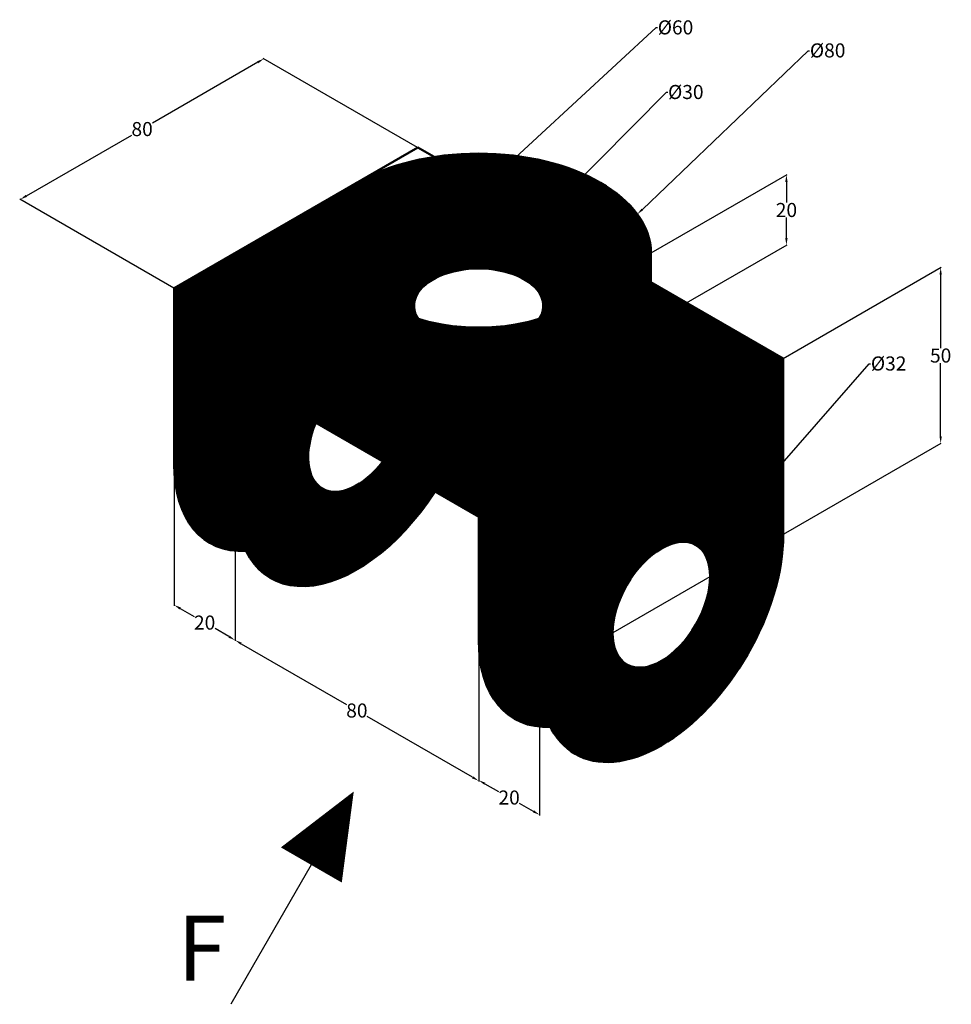
# Model space of a CAD drawing. Units: millimetres. Extents: x -475 to 40, y -900 to -205.
# Tile 1 of 1: x -318.9 to -53.9, y -485 to -205. Entities that reach past the tile are written whole.
import ezdxf
from ezdxf import colors
from ezdxf.entities.mleader import LeaderData, LeaderLine
from ezdxf.math import Vec2, Vec3

# ---------------------------------------------------------------- set-up
doc = ezdxf.new("R2010")
doc.units = ezdxf.units.MM
doc.header["$MEASUREMENT"] = 0
for name, color, linetype, lineweight in [('M-ANNO-SYMB', 2, 'Continuous', 25), ('M-DIMS', 2, 'Continuous', 25), ('M-HATC', 8, 'Continuous', 18), ('M-OUTL', 7, 'Continuous', 50), ('M-TEXT', 7, 'Continuous', 25)]:
    doc.layers.add(name, color=color, linetype=linetype, lineweight=lineweight)
doc.styles.get("Standard").update_dxf_attribs({"font": 'arial.ttf'})
doc.dimstyles.get("Standard").update_dxf_attribs({"dimtxt": 4, "dimasz": 2, "dimexe": 0.18, "dimexo": 0.0625, "dimgap": 0.09, "dimtad": 0, "dimtih": 1, "dimtoh": 1, "dimdec": 0, "dimzin": 0, "dimdsep": 46, "dimtxsty": 'Standard', "dimcen": 0.09, "dimadec": 0, "dimazin": 0, "dimtfac": 1, "dimtdec": 0, "dimtofl": 0, "dimtmove": 0, "dimatfit": 3, "dimfxl": 1, "dimtolj": 1, "dimtzin": 0, "dimarcsym": 0})

# ---------------------------------------------------------------- blocks, each defined once
blk = doc.blocks.new('*D1')
at = {"layer": 'Defpoints', "color": 0, "transparency": 16777216}
for p in [(-56.94566817318142, -325.4711766746398), (-171.0183611883869, -341.3310766941546), (-171.0183611883869, -391.3310766941547)]:
    blk.add_point(p, dxfattribs=at)
at = {"layer": 'M-DIMS', "color": 0, "lineweight": -2, "transparency": 16777216}
for p, q in [((-170.9558611883869, -341.2949923023302), (-56.76566817318142, -275.3672536261856)), ((-56.94566817318142, -277.4711766746397), (-56.94566817318142, -298.3388847237529)), ((-56.94566817318142, -323.4711766746398), (-56.94566817318142, -302.6034686255265)), ((-170.9558611883869, -391.2949923023303), (-56.76566817318141, -325.3672536261856))]:
    blk.add_line(p, q, dxfattribs=at)
at = {"layer": 'M-DIMS', "color": 0, "transparency": 16777216}
for points in [[(-57.27900150651476, -277.4711766746397), (-56.61233483984808, -277.4711766746397), (-56.94566817318142, -275.4711766746397)], [(-57.27900150651475, -323.4711766746398), (-56.61233483984808, -323.4711766746398), (-56.94566817318142, -325.4711766746398)]]:
    blk.add_solid(points, dxfattribs=at)
at = {"layer": 'M-DIMS', "color": 0, "transparency": 16777216, "insert": (-56.9456681731815, -300.4711766746396), "char_height": 4, "attachment_point": 5}
blk.add_mtext('\\A1;50', dxfattribs=at)
blk = doc.blocks.new('*D2')
at = {"layer": 'Defpoints', "color": 0, "transparency": 16777216}
for p in [(-188.3388692640756, -346.3310766941546), (-171.0183611883868, -356.164245815369), (-171.0183611883869, -431.07672200079)]:
    blk.add_point(p, dxfattribs=at)
at = {"layer": 'M-DIMS', "color": 0, "lineweight": -2, "transparency": 16777216}
for p, q in [((-188.3388692640756, -346.402946369226), (-188.3388692640757, -421.4505375437814)), ((-171.0183611883868, -356.2361154904404), (-171.0183611883869, -431.2837066649958)), ((-186.5996099745945, -422.2309621786778), (-182.6608389642941, -424.4670744973681)), ((-172.757620477868, -430.0893127016877), (-176.6963914881685, -427.8532003829974))]:
    blk.add_line(p, q, dxfattribs=at)
at = {"layer": 'M-DIMS', "color": 0, "transparency": 16777216}
for points in [[(-186.4350417580775, -421.941085630431), (-186.7641781911116, -422.5208387269247), (-188.3388692640757, -421.2435528795755)], [(-172.5930522613509, -429.7994361534409), (-172.922188694385, -430.3791892499345), (-171.0183611883869, -431.07672200079)]]:
    blk.add_solid(points, dxfattribs=at)
at = {"layer": 'M-DIMS', "color": 0, "transparency": 16777216, "insert": (-179.6786152262312, -426.1601374401827), "char_height": 4, "attachment_point": 5}
blk.add_mtext('\\A1;20', dxfattribs=at)
blk = doc.blocks.new('*D3')
at = {"layer": 'Defpoints', "color": 0, "transparency": 16777216}
for p in [(-257.6209015668307, -341.3310766941545), (-257.6209015668307, -381.4107159153928), (-188.3388692640756, -381.3310766941545)]:
    blk.add_point(p, dxfattribs=at)
at = {"layer": 'M-DIMS', "color": 0, "lineweight": -2, "transparency": 16777216}
for p, q in [((-257.6209015668307, -341.4032454778032), (-257.6209015668307, -381.618562012301)), ((-255.8888507592618, -382.4107159153927), (-225.9307312544708, -399.7070442758987)), ((-188.3388692640756, -381.4032454778032), (-188.3388692640756, -421.618562012301)), ((-190.0709200716445, -420.4107159153927), (-220.0290395764354, -403.1143875548867))]:
    blk.add_line(p, q, dxfattribs=at)
at = {"layer": 'M-DIMS', "color": 0, "transparency": 16777216}
for points in [[(-255.7221840925951, -382.1220407807979), (-256.0555174259284, -382.6993910499875), (-257.6209015668307, -381.4107159153928)], [(-189.9042534049778, -420.1220407807979), (-190.2375867383111, -420.6993910499875), (-188.3388692640756, -421.4107159153927)]]:
    blk.add_solid(points, dxfattribs=at)
at = {"layer": 'M-DIMS', "color": 0, "transparency": 16777216, "insert": (-222.9798854154531, -401.4107159153927), "char_height": 4, "attachment_point": 5}
blk.add_mtext('\\A1;80', dxfattribs=at)
blk = doc.blocks.new('*D4')
at = {"layer": 'Defpoints', "color": 0, "transparency": 16777216}
for p in [(-274.9414096425195, -331.3310766941545), (-257.6209015668307, -341.3310766941545), (-274.9414096425194, -371.4107159153929)]:
    blk.add_point(p, dxfattribs=at)
at = {"layer": 'M-DIMS', "color": 0, "lineweight": -2, "transparency": 16777216}
for p, q in [((-274.9414096425195, -331.4032454778032), (-274.9414096425194, -371.6185620123011)), ((-257.6209015668307, -341.4032454778032), (-257.6209015668307, -381.6185620123011)), ((-273.2093588349505, -372.4107159153929), (-269.2633793427378, -374.6889282374386)), ((-259.3529523743995, -380.4107159153929), (-263.2989318666123, -378.1325035933471))]:
    blk.add_line(p, q, dxfattribs=at)
at = {"layer": 'M-DIMS', "color": 0, "transparency": 16777216}
for points in [[(-273.0426921682839, -372.122040780798), (-273.3760255016172, -372.6993910499877), (-274.9414096425194, -371.4107159153929)], [(-259.1862857077329, -380.122040780798), (-259.5196190410662, -380.6993910499877), (-257.6209015668307, -381.4107159153929)]]:
    blk.add_solid(points, dxfattribs=at)
at = {"layer": 'M-DIMS', "color": 0, "transparency": 16777216, "insert": (-266.2811556046751, -376.4107159153929), "char_height": 4, "attachment_point": 5}
blk.add_mtext('\\A1;20', dxfattribs=at)
blk = doc.blocks.new('*D5')
at = {"layer": 'Defpoints', "color": 0, "transparency": 16777216}
for p in [(-249.4178865535401, -216.0670896202445), (-205.6593773397644, -241.3310766941545), (-274.9414096425195, -281.3310766941545)]:
    blk.add_point(p, dxfattribs=at)
at = {"layer": 'M-DIMS', "color": 0, "lineweight": -2, "transparency": 16777216}
for p, q in [((-251.149937361109, -217.0670896202445), (-281.1080568658999, -234.3634179807505)), ((-205.7218773397644, -241.2949923023302), (-249.5978865535401, -215.9631665717903)), ((-316.9678680487263, -255.0670896202445), (-287.0097485439354, -237.7707612597385)), ((-275.0039096425195, -281.2949923023302), (-318.8799188562951, -255.9631665717903))]:
    blk.add_line(p, q, dxfattribs=at)
at = {"layer": 'M-DIMS', "color": 0, "transparency": 16777216}
for points in [[(-251.3166040277756, -216.7784144856497), (-250.9832706944423, -217.3557647548393), (-249.4178865535401, -216.0670896202445)], [(-317.134534715393, -254.7784144856497), (-316.8012013820596, -255.3557647548393), (-318.6999188562952, -256.0670896202445)]]:
    blk.add_solid(points, dxfattribs=at)
at = {"layer": 'M-DIMS', "color": 0, "transparency": 16777216, "insert": (-284.0589027049176, -236.0670896202445), "char_height": 4, "attachment_point": 5}
blk.add_mtext('\\A1;80', dxfattribs=at)
blk = doc.blocks.new('*D6')
at = {"layer": 'Defpoints', "color": 0, "transparency": 16777216}
for p in [(-139.3490744084121, -271.3310766941546), (-100.8156650904446, -269.0838024516319), (-139.3490744084121, -291.3310766941546)]:
    blk.add_point(p, dxfattribs=at)
at = {"layer": 'M-DIMS', "color": 0, "lineweight": -2, "transparency": 16777216}
for p, q in [((-139.2865744084121, -271.2949923023302), (-100.6356650904446, -248.9798794031778)), ((-100.8156650904446, -251.0838024516319), (-100.8156650904446, -256.9515105007451)), ((-100.8156650904446, -267.0838024516319), (-100.8156650904446, -261.2160944025187)), ((-139.2865744084121, -291.2949923023303), (-100.6356650904446, -268.9798794031777))]:
    blk.add_line(p, q, dxfattribs=at)
at = {"layer": 'M-DIMS', "color": 0, "transparency": 16777216}
for points in [[(-101.148998423778, -251.0838024516319), (-100.4823317571113, -251.0838024516319), (-100.8156650904446, -249.0838024516319)], [(-101.148998423778, -267.0838024516319), (-100.4823317571113, -267.0838024516319), (-100.8156650904446, -269.0838024516319)]]:
    blk.add_solid(points, dxfattribs=at)
at = {"layer": 'M-DIMS', "color": 0, "transparency": 16777216, "insert": (-100.8156650904447, -259.0838024516318), "char_height": 4, "attachment_point": 5}
blk.add_mtext('\\A1;20', dxfattribs=at)

msp = doc.modelspace()

# ---------------------------------------------------------------- hatches: boundary and pattern name
at = {"layer": 'M-HATC'}
h = msp.add_hatch(dxfattribs=at)
h.set_pattern_fill('ANSI31', color=256)
h.set_pattern_definition([(45, (-328.3383552602089, -427.0710071446905), (-0.0883883476483185, 0.0883883476483185), [])])
edge = h.paths.add_edge_path()
edge.add_ellipse((-188.3388692640756, -271.3310766941545), major_axis=(-48.98979485566356, 3.1e-15), ratio=0.577350269189626, start_angle=330, end_angle=360, ccw=False)
edge.add_line((-222.9798854154533, -251.3310766941545), (-274.9414096425195, -281.3310766941545))
edge.add_line((-274.9414096425195, -281.3310766941545), (-222.979885415453, -311.3310766941546))
edge.add_ellipse((-188.3388692640756, -291.3310766941545), major_axis=(-48.98979485566356, 3.1e-15), ratio=0.577350269189626, start_angle=0, end_angle=30, ccw=False)
edge.add_line((-237.3286641197392, -291.3310766941545), (-237.3286641197392, -271.3310766941545))
edge = h.paths.add_edge_path()
edge.add_line((-101.7363288856317, -301.3310766941545), (-139.349074408412, -279.6153479416164))
edge.add_line((-139.349074408412, -279.6153479416164), (-139.349074408412, -291.3310766941543))
edge.add_ellipse((-188.3388692640756, -291.3310766941545), major_axis=(-48.98979485566356, 3.1e-15), ratio=0.577350269189626, start_angle=30, end_angle=180, ccw=False)
edge.add_line((-222.9798854154533, -311.3310766941544), (-171.0183611883868, -341.3310766941545))
edge.add_line((-171.0183611883868, -341.3310766941545), (-101.7363288856317, -301.3310766941545))
edge = h.paths.add_edge_path()
edge.add_ellipse((-188.3388692640756, -291.3310766941545), major_axis=(-48.98979485566356, 3.1e-15), ratio=0.577350269189626, start_angle=30.00000000000002, end_angle=180)
edge.add_line((-139.349074408412, -291.3310766941543), (-139.349074408412, -279.6153479416164))
edge.add_line((-139.349074408412, -279.6153479416164), (-139.349074408412, -271.3310766941544))
edge.add_ellipse((-188.3388692640756, -271.3310766941545), major_axis=(-48.98979485566356, 3.1e-15), ratio=0.577350269189626, start_angle=0, end_angle=180, ccw=False)
edge.add_line((-237.3286641197392, -271.3310766941545), (-237.3286641197392, -291.3310766941545))
edge.add_ellipse((-188.3388692640756, -291.3310766941545), major_axis=(-48.98979485566356, 3.1e-15), ratio=0.577350269189626, start_angle=0, end_angle=30.00000000000002)
edge = h.paths.add_edge_path()
edge.add_ellipse((-188.3388692640756, -271.3310766941545), major_axis=(-48.98979485566356, 3.1e-15), ratio=0.577350269189626, start_angle=3.6e-15, end_angle=180)
edge.add_ellipse((-188.3388692640756, -271.3310766941545), major_axis=(-48.98979485566356, 3.1e-15), ratio=0.577350269189626, start_angle=180, end_angle=216.4273398800309)
edge.add_line((-158.1530337662851, -249.0539184724817), (-164.3185950845215, -255.2788034559799))
edge.add_ellipse((-188.3388692640756, -271.3310766941545), major_axis=(-36.74234614174767, 1.5e-15), ratio=0.577350269189626, start_angle=167.6900113356715, end_angle=213.7540221323888, ccw=False)
edge.add_ellipse((-188.3388692640756, -271.3310766941545), major_axis=(-36.74234614174767, 1.5e-15), ratio=0.577350269189626, start_angle=132.5057290121876, end_angle=167.6900113356715, ccw=False)
edge.add_ellipse((-188.3388692640756, -271.3310766941545), major_axis=(-36.74234614174767, 1.5e-15), ratio=0.577350269189626, start_angle=47.4942709878124, end_angle=132.5057290121876, ccw=False)
edge.add_ellipse((-188.3388692640756, -271.3310766941545), major_axis=(-36.74234614174767, 1.5e-15), ratio=0.577350269189626, start_angle=12.309988664328614, end_angle=47.4942709878124, ccw=False)
edge.add_ellipse((-188.3388692640756, -271.3310766941545), major_axis=(-36.74234614174767, 1.5e-15), ratio=0.577350269189626, start_angle=213.7540221323888, end_angle=372.30998866432856, ccw=False)
edge.add_line((-164.3185950845215, -255.2788034559799), (-158.1530337662851, -249.0539184724817))
edge.add_ellipse((-188.3388692640756, -271.3310766941545), major_axis=(-48.98979485566356, 3.1e-15), ratio=0.577350269189626, start_angle=216.4273398800309, end_angle=248.418359243648)
edge.add_ellipse((-188.3388692640756, -271.3310766941545), major_axis=(-48.98979485566356, 3.1e-15), ratio=0.577350269189626, start_angle=248.418359243648, end_angle=294.8960906389828)
edge.add_ellipse((-188.3388692640756, -271.3310766941545), major_axis=(-48.98979485566356, 3.1e-15), ratio=0.577350269189626, start_angle=294.8960906389828, end_angle=330)
edge.add_ellipse((-188.3388692640756, -271.3310766941545), major_axis=(-48.98979485566356, 3.1e-15), ratio=0.577350269189626, start_angle=330, end_angle=360)
edge = h.paths.add_edge_path(flags=17)
edge.add_ellipse((-188.3388692640756, -271.3310766941545), major_axis=(-36.74234614174767, 1.5e-15), ratio=0.577350269189626, start_angle=213.7540221323888, end_angle=372.3099886643286)
edge.add_ellipse((-188.3388692640756, -286.3310766941545), major_axis=(-36.74234614174767, 1.5e-15), ratio=0.577350269189626, start_angle=236.92679235372322, end_angle=347.69001133567144, ccw=False)
edge.add_line((-175.4080661358342, -266.474974941304), (-164.3185950845215, -255.27880345598))
edge = h.paths.add_edge_path(flags=17)
edge.add_ellipse((-188.3388692640756, -271.3310766941545), major_axis=(-36.74234614174767, 1.5e-15), ratio=0.577350269189626, start_angle=167.6900113356714, end_angle=213.7540221323888)
edge.add_line((-164.3185950845215, -255.2788034559799), (-175.4080661358342, -266.474974941304))
edge.add_ellipse((-188.3388692640756, -286.3310766941545), major_axis=(-36.74234614174767, 1.5e-15), ratio=0.577350269189626, start_angle=192.3099886643282, end_angle=236.9267923537231, ccw=False)
edge = h.paths.add_edge_path(flags=17)
edge.add_ellipse((-188.3388692640756, -286.3310766941545), major_axis=(-36.74234614174767, 1.5e-15), ratio=0.577350269189626, start_angle=192.3099886643282, end_angle=236.9267923537231)
edge.add_ellipse((-188.3388692640756, -286.3310766941545), major_axis=(-36.74234614174767, 1.5e-15), ratio=0.577350269189626, start_angle=236.9267923537231, end_angle=347.6900113356714)
edge.add_ellipse((-188.3388692640756, -271.3310766941545), major_axis=(-36.74234614174767, 1.5e-15), ratio=0.577350269189626, start_angle=12.30998866432856, end_angle=47.49427098781236)
edge.add_ellipse((-188.3388692640756, -286.3310766941545), major_axis=(-18.37117307087383, 1.5e-15), ratio=0.577350269189626, start_angle=167.6900113356715, end_angle=372.30998866432856, ccw=False)
edge.add_ellipse((-188.3388692640756, -271.3310766941545), major_axis=(-36.74234614174767, 1.5e-15), ratio=0.577350269189626, start_angle=132.5057290121876, end_angle=167.6900113356714)
edge = h.paths.add_edge_path()
edge.add_line((-101.7363288856317, -301.3310766941545), (-171.0183611883868, -341.3310766941545))
edge.add_line((-171.0183611883868, -341.3310766941545), (-171.0183611883868, -391.3310766941542))
edge.add_ellipse((-136.3773450370093, -371.3310766941545), major_axis=(-24.49489742783177, -42.42640687119285), ratio=0.577350269189626, start_angle=329.9999999999999, end_angle=347.6900113356714)
edge.add_ellipse((-136.3773450370093, -371.3310766941545), major_axis=(-24.49489742783177, -42.42640687119285), ratio=0.577350269189626, start_angle=347.6900113356714, end_angle=509.9999999999999)
edge.add_line((-101.7363288856317, -351.3310766941553), (-101.7363288856317, -301.3310766941545))
edge = h.paths.add_edge_path(flags=16)
edge.add_ellipse((-136.3773450370093, -371.3310766941545), major_axis=(-9.797958971132706, -16.97056274847714), ratio=0.577350269189626, start_angle=0, end_angle=360)
edge = h.paths.add_edge_path()
edge.add_line((-222.9798854154533, -311.3310766941544), (-274.9414096425195, -281.3310766941545))
edge.add_line((-274.9414096425195, -281.3310766941545), (-274.9414096425195, -331.3310766941543))
edge.add_ellipse((-240.3003934911419, -311.3310766941545), major_axis=(-24.49489742783177, -42.42640687119285), ratio=0.577350269189626, start_angle=329.9999999999999, end_angle=372.3099886642788)
edge.add_ellipse((-222.9798854154532, -321.3310766941545), major_axis=(-24.49489742783177, -42.42640687119285), ratio=0.577350269189626, start_angle=329.99999999999994, end_angle=347.69001133567144, ccw=False)
edge.add_line((-257.6209015668307, -341.3310766941541), (-257.6209015668307, -306.3310766941545))
edge.add_line((-257.6209015668307, -306.3310766941545), (-188.3388692640756, -346.3310766941545))
edge.add_line((-188.3388692640756, -346.3310766941545), (-188.3388692640756, -381.3310766941543))
edge.add_ellipse((-153.697853112698, -361.3310766941545), major_axis=(-24.49489742783177, -42.42640687119285), ratio=0.577350269189626, start_angle=329.9999999999999, end_angle=372.3099886642788)
edge.add_ellipse((-136.3773450370093, -371.3310766941545), major_axis=(-24.49489742783177, -42.42640687119285), ratio=0.577350269189626, start_angle=329.99999999999994, end_angle=347.69001133567144, ccw=False)
edge.add_line((-171.0183611883868, -391.331076694154), (-171.0183611883868, -341.3310766941545))
edge.add_line((-171.0183611883868, -341.3310766941545), (-222.9798854154533, -311.3310766941544))
edge = h.paths.add_edge_path(flags=17)
edge.add_ellipse((-222.9798854154532, -321.3310766941545), major_axis=(-24.49489742783177, -42.42640687119285), ratio=0.577350269189626, start_angle=347.6900113356714, end_angle=441.2623174267488)
edge.add_line((-200.7459223049853, -339.1678612811353), (-215.5891914981061, -330.5980958168329))
edge.add_ellipse((-222.9798854154532, -321.3310766941545), major_axis=(-9.797958971132706, -16.97056274847714), ratio=0.577350269189626, start_angle=291.4267091514603, end_angle=428.5732908485397, ccw=False)
edge.add_line((-234.7007063517224, -319.564057571476), (-257.6209015668307, -306.3310766941545))
edge.add_line((-257.6209015668307, -306.3310766941545), (-257.6209015668307, -341.3310766941541))
edge.add_ellipse((-222.9798854154532, -321.3310766941545), major_axis=(-24.49489742783177, -42.42640687119285), ratio=0.577350269189626, start_angle=329.9999999999999, end_angle=347.6900113356714)

# ---------------------------------------------------------------- linework, layer by layer
at = {"layer": 'M-ANNO-SYMB'}
msp.add_line((-235.9352353405691, -445.3403348579658), (-258.8089789745049, -484.9588209912478), dxfattribs=at)
msp.add_lwpolyline([(-235.9352353405691, -445.3403348579658, 20, 0, 0), (-223.8609380176139, -424.4270384289145, 0, 0, 0)], format="xyseb", dxfattribs=at)
at = {"layer": 'M-OUTL'}
for p, q in [((-274.9414096425195, -281.3310766941545), (-205.6593773397644, -241.3310766941545)), ((-205.6593773397644, -241.3310766941545), (-201.0183611883868, -244.0105686184658)), ((-237.3286641197392, -271.3310766941545), (-237.3286641197392, -291.3310766941545)), ((-139.349074408412, -271.3310766941545), (-139.349074408412, -291.3310766941545)), ((-139.349074408412, -279.6153479416164), (-101.7363288856317, -301.3310766941545)), ((-171.0183611883868, -341.3310766941545), (-274.9414096425195, -281.3310766941545)), ((-274.9414096425195, -281.3310766941545), (-274.9414096425195, -331.3310766941545)), ((-171.0183611883868, -341.3310766941545), (-101.7363288856317, -301.3310766941545)), ((-101.7363288856317, -301.3310766941545), (-101.7363288856317, -351.3310766941545)), ((-257.6209015668307, -306.3310766941545), (-257.6209015668307, -341.3310766941545)), ((-188.3388692640756, -346.3310766941545), (-257.6209015668307, -306.3310766941545)), ((-171.0183611883868, -341.3310766941545), (-171.0183611883868, -391.3310766941545)), ((-188.3388692640756, -346.3310766941545), (-188.3388692640756, -381.3310766941545))]:
    msp.add_line(p, q, dxfattribs=at)
for centre, major_axis in [((-188.3388692640756, -271.3310766941545), (-48.98979485566356, 3.1e-15)), ((-188.3388692640756, -271.3310766941545), (-36.74234614174767, 1.5e-15)), ((-136.3773450370093, -371.3310766941545), (-9.797958971132706, -16.97056274847714))]:
    msp.add_ellipse(centre, major_axis=major_axis, ratio=0.577350269189626, dxfattribs=at)
for centre, major_axis, start_param, end_param in [((-188.3388692640756, -286.3310766941545), (-36.74234614174767, 1.5e-15), 3.50295977749649, 5.921818183272877), ((-188.3388692640756, -286.3310766941545), (-18.37117307087383, 1.5e-15), 2.780225529683085, 6.644552431086293), ((-188.3388692640756, -291.3310766941545), (-48.98979485566356, 3.1e-15), 0, 3.141592653589793), ((-222.9798854154532, -321.3310766941545), (-9.797958971132706, -16.97056274847714), 4.935198815711101, 7.631171798648071), ((-240.3003934911419, -311.3310766941545), (-24.49489742783177, -42.42640687119285), 5.497787143782137, 6.644552431084916), ((-222.9798854154532, -321.3310766941545), (-24.49489742783177, -42.42640687119285), 5.497787143782137, 7.765477790830463), ((-136.3773450370093, -371.3310766941545), (-24.49489742783177, -42.42640687119285), 5.497787143782137, 8.63937979737193), ((-153.697853112698, -361.3310766941545), (-24.49489742783177, -42.42640687119285), 5.497787143782137, 6.644552431084916)]:
    msp.add_ellipse(centre, major_axis=major_axis, ratio=0.577350269189626, start_param=start_param, end_param=end_param, dxfattribs=at)

# ---------------------------------------------------------------- texts
at = {"layer": 'M-TEXT'}
msp.add_text('F', height=18.43271151920555, dxfattribs=at).set_placement((-274.0271530944519, -478.2182776550038))

# ---------------------------------------------------------------- dimensions: what is measured, and where the dimension line sits
at = {"layer": 'M-DIMS'}
for p1, p2, distance, picture, middle in [((-274.9414096425195, -281.3310766941545), (-205.6593773397644, -241.3310766941545), 43.75850921377558, '*D5', (-284.0589027049176, -236.0670896202445)), ((-139.349074408412, -271.3310766941545), (-139.349074408412, -291.3310766941545), 38.53340931796741, '*D6', (-100.8156650904447, -259.0838024516318)), ((-171.0183611883868, -341.3310766941545), (-171.0183611883868, -391.3310766941545), 114.07269301520537, '*D1', (-56.9456681731815, -300.4711766746396)), ((-257.6209015668307, -341.3310766941545), (-274.9414096425195, -331.3310766941545), 34.70998574010759, '*D4', (-266.2811556046751, -376.4107159153929)), ((-188.3388692640756, -381.3310766941545), (-257.6209015668307, -341.3310766941545), 34.70998574010754, '*D3', (-222.9798854154531, -401.4107159153927)), ((-188.3388692640756, -346.3310766941545), (-171.0183611883868, -356.1642458153689), -65.14611005176354, '*D2', (-179.6786152262312, -426.1601374401827))]:
    dim = msp.add_aligned_dim(p1=p1, p2=p2, distance=distance, dimstyle='Standard', override={"dimclrd": 0, "dimclre": 0, "dimclrt": 0}, dxfattribs=at)
    dim.commit()
    dim.dimension.update_dxf_attribs({"geometry": picture, "text_midpoint": middle})

# ---------------------------------------------------------------- leaders
ml = msp.add_multileader_mtext('Standard', dxfattribs=at)
ml.set_content('%%C60', color=256)
ml.set_leader_properties()
ml.build(insert=Vec2(0, 0))
ml.multileader.update_dxf_attribs({"dogleg_length": 0.36, "arrow_head_size": 2})
ctx = ml.context
ctx.base_point, ctx.arrow_head_size, ctx.landing_gap_size, ctx.plane_origin = Vec3(-137.498386941451, -207.2357888024651), 2, 0.09, Vec3(-184.4533055337964, -250.2368247559452)
notes = []
notes.append((ctx, [(0, (1, 1, 0), (-137.858386941451, -207.2357888024651), (1, 0), 0.36, [(0, [(-184.4533055337964, -250.2368247559452)], 0, [])])]))
ctx.mtext.insert, ctx.mtext.flow_direction = Vec3(-137.408386941451, -205.1552976701323), 5
ml = msp.add_multileader_mtext('Standard', dxfattribs=at)
ml.set_content('%%C80', color=256)
ml.set_leader_properties()
ml.build(insert=Vec2(0, 0))
ml.multileader.update_dxf_attribs({"dogleg_length": 0.36, "arrow_head_size": 2})
ctx = ml.context
ctx.base_point, ctx.arrow_head_size, ctx.landing_gap_size, ctx.plane_origin = Vec3(-94.2272415017568, -213.7873324322215), 2, 0.09, Vec3(-143.2340961519432, -260.2923653789229)
notes.append((ctx, [(0, (1, 1, 0), (-94.58724150175681, -213.7873324322215), (1, 0), 0.36, [(0, [(-143.2340961519369, -260.2923653789316)], 0, [])])]))
ctx.mtext.insert, ctx.mtext.flow_direction = Vec3(-94.1372415017568, -211.7068412998886), 5
ml = msp.add_multileader_mtext('Standard', dxfattribs=at)
ml.set_content('%%C30', color=256)
ml.set_leader_properties()
ml.build(insert=Vec2(0, 0))
ml.multileader.update_dxf_attribs({"dogleg_length": 0.36, "arrow_head_size": 2})
ctx = ml.context
ctx.base_point, ctx.arrow_head_size, ctx.landing_gap_size, ctx.plane_origin = Vec3(-134.5767980746226, -225.6143013036554), 2, 0.09, Vec3(-184.769601774938, -275.9265852026401)
notes.append((ctx, [(0, (1, 1, 0), (-134.9367980746226, -225.6143013036554), (1, 0), 0.36, [(0, [(-184.769601774938, -275.9265852026401)], 0, [])])]))
ctx.mtext.insert, ctx.mtext.flow_direction = Vec3(-134.4867980746226, -223.5338101713225), 5
ml = msp.add_multileader_mtext('Standard', dxfattribs=at)
ml.set_content('%%C32', color=256)
ml.set_leader_properties()
ml.build(insert=Vec2(0, 0))
ml.multileader.update_dxf_attribs({"dogleg_length": 0.36, "arrow_head_size": 2})
ctx = ml.context
ctx.base_point, ctx.arrow_head_size, ctx.landing_gap_size, ctx.plane_origin = Vec3(-76.88150865255433, -302.8146716772694), 2, 0.09, Vec3(-124.2355850813548, -356.6114961047599)
notes.append((ctx, [(0, (1, 1, 0), (-77.24150865255433, -302.8146716772694), (1, 0), 0.36, [(0, [(-124.2355850813548, -356.6114961047599)], 0, [])])]))
ctx.mtext.insert, ctx.mtext.flow_direction = Vec3(-76.79150865255433, -300.7341805449365), 5
for ctx, leaders in notes:
    for number, flags, end, landing, length, lines in leaders:
        leader = LeaderData()
        leader.index, (leader.has_last_leader_line, leader.has_dogleg_vector, leader.attachment_direction) = number, flags
        leader.last_leader_point, leader.dogleg_vector, leader.dogleg_length = Vec3(end), Vec3(landing), length
        for number, points, colour, breaks in lines:
            line = LeaderLine()
            line.index, line.vertices, line.color, line.breaks = number, Vec3.list(points), colors.encode_raw_color(colour), breaks
            leader.lines.append(line)
        ctx.leaders.append(leader)

doc.saveas('drawing.dxf')
